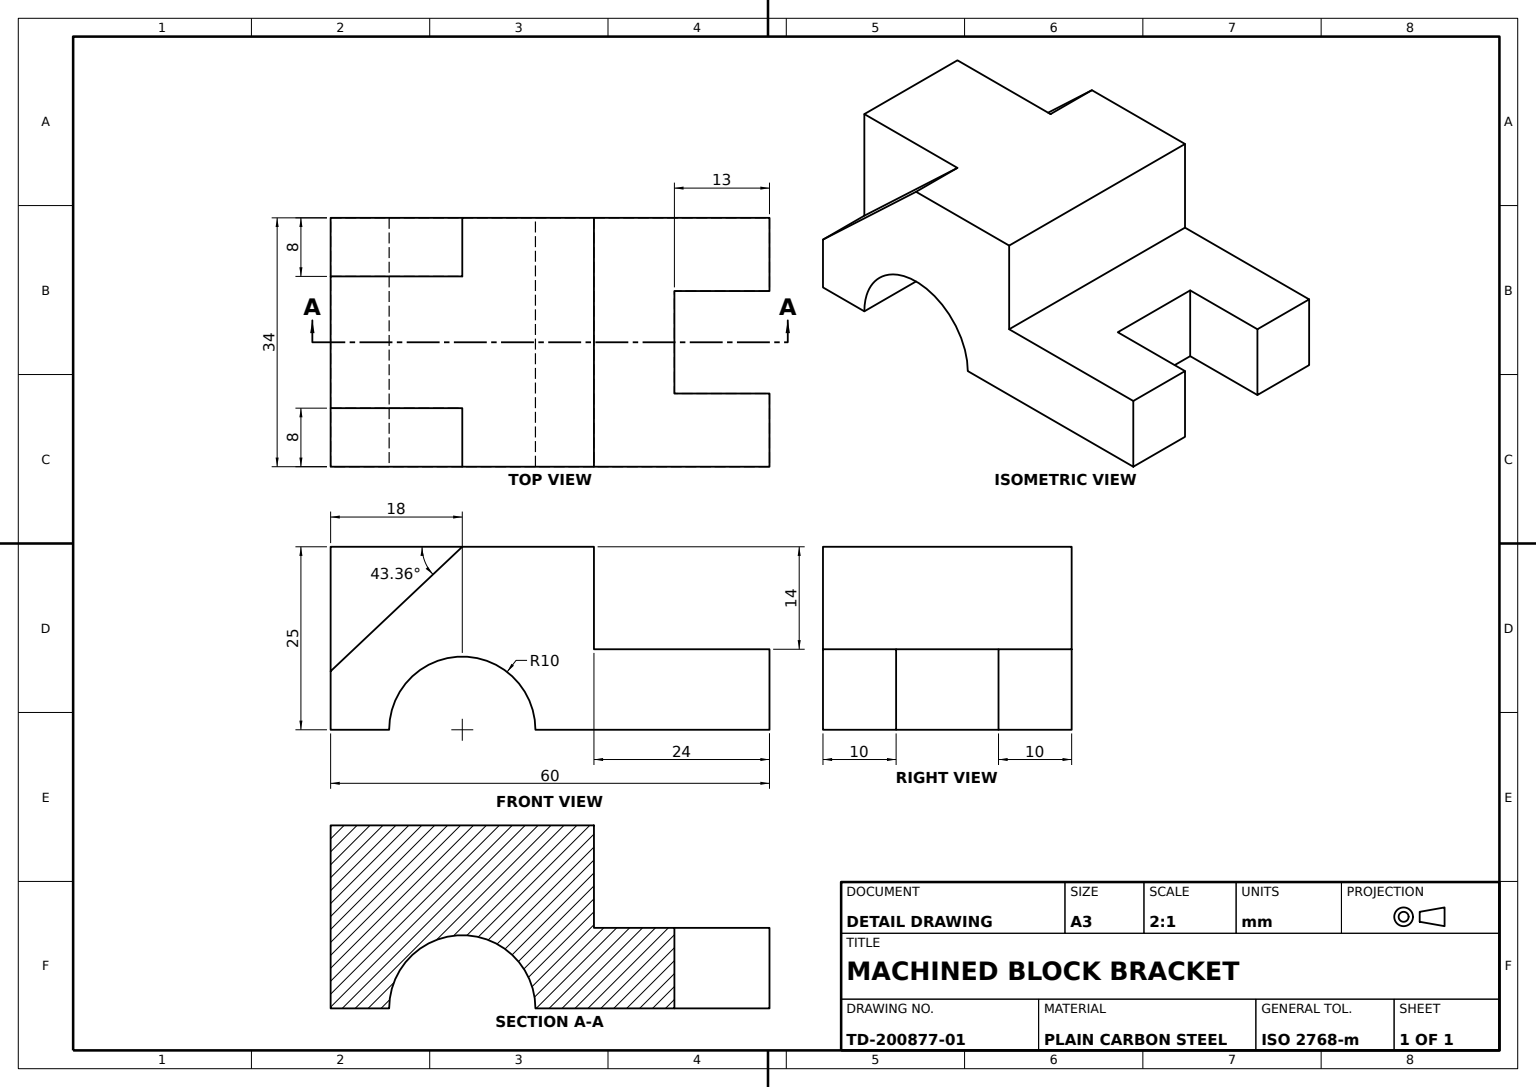
from build123d import *

# Parameters (mm, degrees)
BLOCK_PROFILE_SKETCH_W       = 60
BLOCK_PROFILE_SKETCH_H       = 25
BASE_BLOCK_DEPTH             = 34
STEP_CUT_PROFILE_SKETCH_W    = 24
STEP_CUT_PROFILE_SKETCH_H    = 14
STEPPED_THROUGH_CUT_DEPTH    = 34
NOTCH_PROFILE_SKETCH_W       = 14
NOTCH_PROFILE_SKETCH_H       = 13
SIDE_NOTCH_THROUGH_CUT_DEPTH = 34
SLOT_18X8_DEPTH_8_DEPTH      = 8
ARCH_RELIEF_CUT_DEPTH        = 8


with BuildPart() as part:
    # Block Profile Sketch → Base Block (new body)
    with BuildSketch(Plane(origin=(0, 0, 0), x_dir=(0, 0, -1), z_dir=(1, 0, 0))):
        Rectangle(BLOCK_PROFILE_SKETCH_W, BLOCK_PROFILE_SKETCH_H)
    extrude(amount=BASE_BLOCK_DEPTH)

    # Step Cut Profile Sketch → Stepped Through Cut (cut)
    with BuildSketch(Plane(origin=(34, 0, 0), x_dir=(0, 0, -1), z_dir=(1, 0, 0))):
        with Locations((18, 5.5)):
            Rectangle(STEP_CUT_PROFILE_SKETCH_W, STEP_CUT_PROFILE_SKETCH_H)
        with BuildLine():
            Line((-22, -12.5), (-2, -12.5))
            ThreePointArc((-2, -12.5), (-12, -2.5), (-22, -12.5))
        make_face()
    extrude(amount=-STEPPED_THROUGH_CUT_DEPTH, mode=Mode.SUBTRACT)

    # Notch Profile Sketch → Side Notch Through Cut (cut)
    with BuildSketch(Plane(origin=(0, 12.5, 0), x_dir=(1, 0, 0), z_dir=(0, 1, 0))):
        with Locations((17, 23.5)):
            Rectangle(NOTCH_PROFILE_SKETCH_W, NOTCH_PROFILE_SKETCH_H)
    extrude(amount=-SIDE_NOTCH_THROUGH_CUT_DEPTH, mode=Mode.SUBTRACT)

    # Slot Sketch → Slot 18x8 Depth 8 (cut)
    with BuildSketch(Plane(origin=(34, 0, 0), x_dir=(0, 0, -1), z_dir=(1, 0, 0))):
        Polygon((-30, 12.5), (-30, -4.5), (-12, 12.5), align=None)
    extrude(amount=-SLOT_18X8_DEPTH_8_DEPTH, mode=Mode.SUBTRACT)

    # Arch Relief Sketch → Arch Relief Cut (cut)
    with BuildSketch(Plane.ZY):
        Polygon((12, 12.5), (30, -4.5), (30, 12.5), align=None)
    extrude(amount=-ARCH_RELIEF_CUT_DEPTH, mode=Mode.SUBTRACT)


solid = part.part
